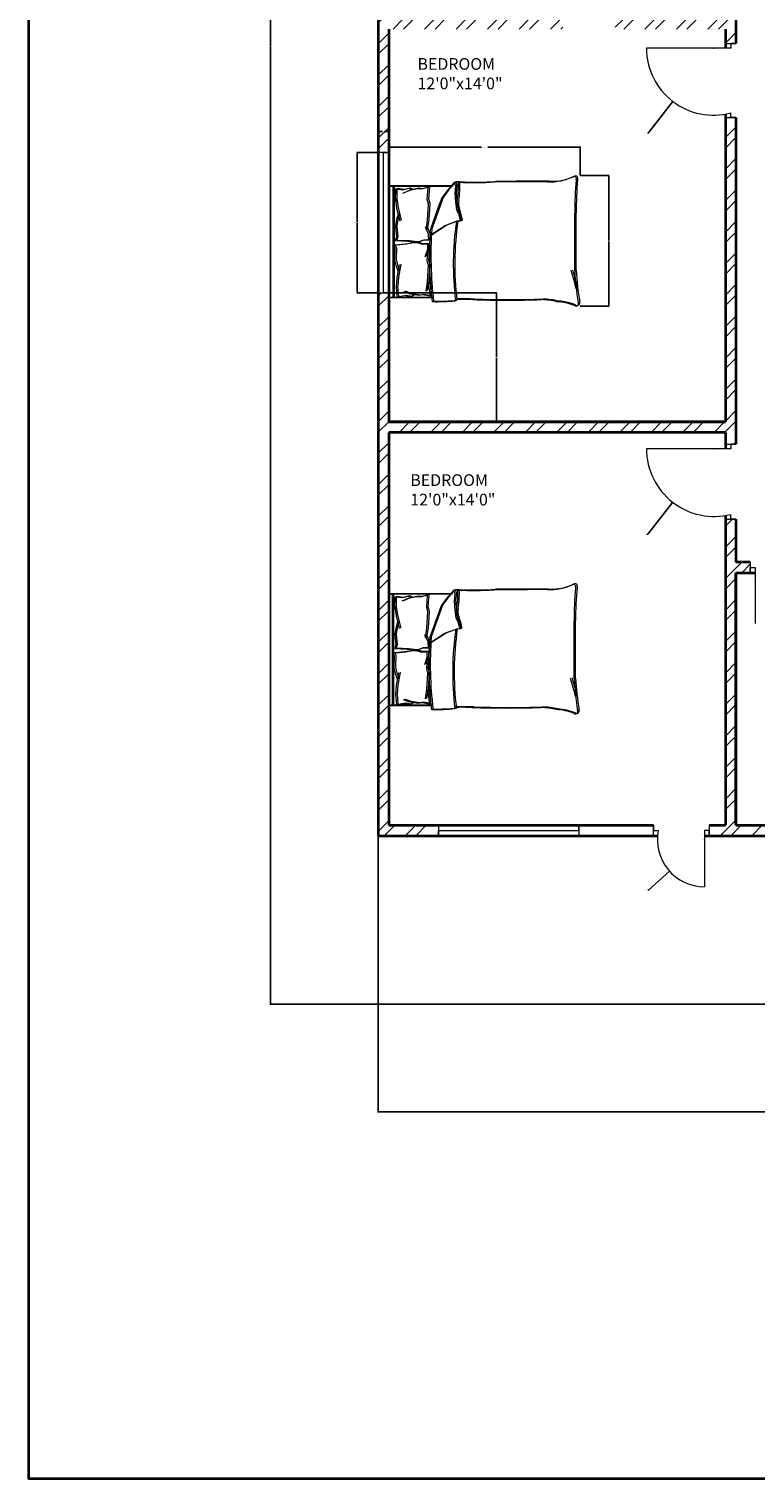
# Model space of a CAD drawing. Units: inches. Extents: x 392 to 1254, y 1207 to 2665.
# Tile 1 of 15: x 392 to 702, y 1207 to 1827. Entities that reach past the tile are written whole.
import ezdxf

# ---------------------------------------------------------------- set-up
doc = ezdxf.new("R2010")
doc.units = ezdxf.units.IN
for name, color, linetype, lineweight in [('A-ANNO-DIMS', 2, 'Continuous', 18), ('A-ANNO-TTLB', 7, 'Continuous', 35), ('A-AREA-IDEN', 7, 'Continuous', 18), ('A-DOOR', 3, 'Continuous', 18), ('A-FURN', 8, 'Continuous', 13), ('A-GLAZ', 4, 'Continuous', 18), ('A-WALL', 7, 'Continuous', 35), ('A-WALL-PATT', 252, 'Continuous', 13)]:
    doc.layers.add(name, color=color, linetype=linetype, lineweight=lineweight)
doc.styles.get("Standard").update_dxf_attribs({"font": 'arial.ttf'})
doc.dimstyles.get("Standard").update_dxf_attribs({"dimtxt": 0.18, "dimasz": 0.18, "dimexe": 0.18, "dimexo": 0.0625, "dimgap": 0.09, "dimtad": 0, "dimtih": 1, "dimtoh": 1, "dimdec": 4, "dimzin": 0, "dimdsep": 46, "dimtxsty": 'Standard', "dimcen": 0.09, "dimadec": 0, "dimazin": 0, "dimtfac": 1, "dimtdec": 4, "dimtofl": 0, "dimtmove": 0, "dimatfit": 3, "dimfxl": 1, "dimtolj": 1, "dimtzin": 0, "dimarcsym": 0})

# ---------------------------------------------------------------- blocks, each defined once
blk = doc.blocks.new('BED-DOUBLE')
for p, q in [((3.47, 63.33), (3.47, 81.44)), ((3.48, 63.33), (3.48, 81.44)), ((3.7, 62.69), (3.7, 80.8)), ((3.7, 62.69), (3.7, 80.8)), ((51.27, 81.44), (51.27, 54.83)), ((51.27, 81.44), (51.27, 54.83)), ((51.49, 81.44), (51.49, 80.8)), ((51.49, 80.8), (51.49, 54.19)), ((51.49, 80.8), (51.49, 54.19)), ((3.47, 79.91), (51.27, 79.91)), ((3.48, 79.91), (51.27, 79.91)), ((3.7, 79.27), (51.49, 79.27)), ((3.7, 79.27), (51.49, 79.27)), ((3.89, 78.13), (4.47, 74.95)), ((3.89, 78.13), (4.47, 74.95)), ((3.9, 78.1), (8.18, 78.43)), ((3.9, 78.1), (8.18, 78.43)), ((4.47, 74.95), (4.04, 72.34)), ((4.47, 74.95), (4.04, 72.34)), ((4.12, 77.49), (4.7, 74.31)), ((4.12, 77.49), (4.7, 74.31)), ((4.13, 77.47), (8.41, 77.79)), ((4.13, 77.47), (8.41, 77.79)), ((5.05, 72.49), (6.06, 75.23)), ((5.05, 72.49), (6.06, 75.23)), ((5.28, 71.85), (6.29, 74.6)), ((5.28, 71.85), (6.29, 74.6)), ((8.18, 78.43), (8.28, 78.42)), ((8.18, 78.43), (8.28, 78.42)), ((8.28, 78.42), (12.11, 78.13)), ((8.28, 78.42), (12.11, 78.13)), ((8.41, 77.79), (8.51, 77.78)), ((8.41, 77.79), (8.51, 77.78)), ((8.51, 77.78), (12.34, 77.49)), ((8.51, 77.78), (12.34, 77.49)), ((12.11, 78.13), (17.6, 77.11)), ((12.11, 78.13), (17.6, 77.11)), ((12.34, 77.49), (17.83, 76.48)), ((12.34, 77.49), (17.83, 76.48)), ((14.85, 77.69), (16.88, 78.42)), ((14.85, 77.69), (16.88, 78.42)), ((15.08, 77.05), (17.11, 77.78)), ((15.08, 77.05), (17.11, 77.78)), ((16.88, 78.42), (19.77, 79.14)), ((16.88, 78.42), (19.77, 79.14)), ((17.11, 77.78), (20, 78.5)), ((17.11, 77.78), (20, 78.5)), ((19.77, 79.14), (20.09, 79.14)), ((19.77, 79.14), (20.09, 79.14)), ((20, 78.5), (20.32, 78.5)), ((20, 78.5), (20.32, 78.5)), ((20.09, 79.14), (24.54, 78.99)), ((20.09, 79.14), (24.54, 78.99)), ((20.32, 78.5), (24.77, 78.35)), ((20.32, 78.5), (24.77, 78.35)), ((24.54, 78.99), (25.98, 79.57)), ((24.54, 78.99), (25.98, 79.57)), ((24.77, 78.35), (26.21, 78.93)), ((24.77, 78.35), (26.21, 78.93)), ((25.98, 79.57), (26.56, 74.22)), ((25.98, 79.57), (26.56, 74.22)), ((26.21, 78.93), (26.79, 73.58)), ((26.21, 78.93), (26.79, 73.58)), ((27.98, 78.95), (27.73, 73.58)), ((27.98, 78.95), (27.73, 73.58)), ((28.21, 78.31), (27.96, 72.94)), ((28.21, 78.31), (27.96, 72.94)), ((29.46, 78.46), (27.98, 78.95)), ((29.46, 78.46), (27.98, 78.95)), ((29.68, 77.82), (28.21, 78.31)), ((29.68, 77.82), (28.21, 78.31)), ((33.88, 78.89), (29.46, 78.46)), ((33.88, 78.89), (29.46, 78.46)), ((34.11, 78.25), (29.68, 77.82)), ((34.11, 78.25), (29.68, 77.82)), ((34.2, 78.91), (33.88, 78.89)), ((34.2, 78.91), (33.88, 78.89)), ((34.43, 78.27), (34.11, 78.25)), ((34.43, 78.27), (34.11, 78.25)), ((37.14, 78.36), (34.2, 78.91)), ((37.14, 78.36), (34.2, 78.91)), ((37.36, 77.73), (34.43, 78.27)), ((37.36, 77.73), (34.43, 78.27)), ((41.91, 78.37), (36.49, 77.02)), ((41.91, 78.37), (36.5, 77.02)), ((42.14, 77.73), (36.72, 76.38)), ((42.14, 77.73), (36.72, 76.38)), ((39.2, 77.77), (37.14, 78.36)), ((39.2, 77.77), (37.14, 78.36)), ((39.43, 77.13), (37.36, 77.73)), ((39.43, 77.13), (37.36, 77.73)), ((45.71, 78.9), (41.91, 78.37)), ((45.71, 78.9), (41.91, 78.37)), ((45.94, 78.26), (42.14, 77.73)), ((45.94, 78.26), (42.14, 77.73)), ((50.11, 78.89), (44.71, 78.98)), ((44.71, 78.98), (45.71, 78.9)), ((50.11, 78.89), (44.71, 78.98)), ((44.71, 78.98), (45.71, 78.9)), ((50.34, 78.25), (44.94, 78.34)), ((44.94, 78.34), (45.94, 78.26)), ((50.34, 78.25), (44.94, 78.34)), ((44.94, 78.34), (45.94, 78.26)), ((49.31, 73.19), (48.13, 75.86)), ((49.31, 73.19), (48.13, 75.86)), ((49.54, 72.55), (48.36, 75.22)), ((49.54, 72.55), (48.36, 75.22)), ((50.11, 78.89), (49.73, 75.67)), ((50.11, 78.89), (49.73, 75.67)), ((49.73, 75.67), (50.33, 73.1)), ((49.73, 75.67), (50.33, 73.1)), ((50.34, 78.25), (49.96, 75.04)), ((50.34, 78.25), (49.96, 75.04)), ((49.96, 75.04), (50.56, 72.47)), ((49.96, 75.04), (50.56, 72.47)), ((4.04, 72.34), (4.62, 71.33)), ((4.04, 72.34), (4.62, 71.33)), ((4.7, 74.31), (4.27, 71.7)), ((4.7, 74.31), (4.27, 71.7)), ((4.27, 71.7), (4.85, 70.69)), ((4.27, 71.7), (4.85, 70.69)), ((4.47, 68.87), (5.05, 72.49)), ((4.47, 68.87), (5.05, 72.49)), ((4.76, 67.28), (4.47, 68.87)), ((4.76, 67.28), (4.47, 68.87)), ((4.7, 68.23), (5.28, 71.85)), ((4.7, 68.23), (5.28, 71.85)), ((4.99, 66.64), (4.7, 68.23)), ((4.99, 66.64), (4.7, 68.23)), ((26.56, 74.22), (27.14, 71.04)), ((26.56, 74.22), (27.14, 71.04)), ((27.14, 69.74), (26.56, 67.86)), ((27.14, 69.74), (26.56, 67.86)), ((26.79, 73.58), (27.37, 70.4)), ((26.79, 73.58), (27.37, 70.4)), ((27.37, 69.1), (26.79, 67.22)), ((27.37, 69.1), (26.79, 67.22)), ((27.14, 71.04), (27.14, 69.74)), ((27.14, 71.04), (27.14, 69.74)), ((27.73, 73.58), (27.35, 70.36)), ((27.73, 73.58), (27.35, 70.36)), ((27.35, 70.36), (27.44, 69.07)), ((27.35, 70.36), (27.44, 69.07)), ((27.37, 70.4), (27.37, 69.1)), ((27.37, 70.4), (27.37, 69.1)), ((27.44, 69.07), (28.13, 67.23)), ((27.44, 69.07), (28.13, 67.23)), ((27.96, 72.94), (27.58, 69.73)), ((27.96, 72.94), (27.58, 69.73)), ((27.58, 69.73), (27.66, 68.43)), ((27.58, 69.73), (27.66, 68.43)), ((27.66, 68.43), (28.36, 66.59)), ((27.66, 68.43), (28.36, 66.59)), ((50.11, 69.61), (49.31, 73.19)), ((50.11, 69.61), (49.31, 73.19)), ((50.34, 68.97), (49.54, 72.55)), ((50.34, 68.97), (49.54, 72.55)), ((50.33, 73.1), (49.81, 72.06)), ((50.33, 73.1), (49.81, 72.06)), ((49.92, 68.01), (50.11, 69.61)), ((49.92, 68.01), (50.11, 69.61)), ((50.56, 72.47), (50.04, 71.42)), ((50.56, 72.47), (50.04, 71.42)), ((50.15, 67.37), (50.34, 68.97)), ((50.15, 67.37), (50.34, 68.97)), ((4.18, 64.1), (4.76, 67.28)), ((4.18, 64.1), (4.76, 67.28)), ((9.28, 64.82), (4.18, 64.1)), ((9.28, 64.82), (4.18, 64.1)), ((4.41, 63.46), (4.99, 66.64)), ((4.41, 63.46), (4.99, 66.64)), ((9.51, 64.19), (4.41, 63.46)), ((9.51, 64.19), (4.41, 63.46)), ((6.38, 65.81), (10.41, 65.15)), ((6.38, 65.81), (10.41, 65.15)), ((6.61, 65.17), (10.64, 64.51)), ((6.61, 65.17), (10.64, 64.51)), ((10.41, 65.15), (9.28, 64.82)), ((10.41, 65.15), (9.28, 64.82)), ((10.64, 64.51), (9.51, 64.19)), ((10.64, 64.51), (9.51, 64.19)), ((10.41, 65.15), (17.42, 64.72)), ((10.41, 65.15), (17.42, 64.72)), ((10.64, 64.51), (17.65, 64.08)), ((10.64, 64.51), (17.65, 64.08)), ((17.42, 64.72), (19.38, 65.27)), ((17.42, 64.72), (19.38, 65.27)), ((17.65, 64.08), (19.61, 64.63)), ((17.65, 64.08), (19.61, 64.63)), ((19.38, 65.27), (24.52, 64.87)), ((19.38, 65.27), (24.52, 64.87)), ((19.61, 64.63), (24.74, 64.23)), ((19.61, 64.63), (24.74, 64.23)), ((24.1, 65.18), (20.96, 66.27)), ((24.1, 65.18), (20.96, 66.27)), ((24.33, 64.54), (21.19, 65.63)), ((24.33, 64.54), (21.19, 65.63)), ((26.56, 65.18), (24.1, 65.18)), ((26.56, 65.18), (24.1, 65.18)), ((26.79, 64.54), (24.33, 64.54)), ((26.79, 64.54), (24.33, 64.54)), ((26.56, 67.86), (26.56, 65.18)), ((26.56, 67.86), (26.56, 65.18)), ((26.79, 67.22), (26.79, 64.54)), ((26.79, 67.22), (26.79, 64.54)), ((28.13, 67.23), (28.3, 64.55)), ((28.13, 67.23), (28.3, 64.55)), ((28.3, 64.55), (30.75, 64.7)), ((28.3, 64.55), (30.75, 64.7)), ((28.36, 66.59), (28.53, 63.91)), ((28.36, 66.59), (28.53, 63.91)), ((28.53, 63.91), (30.98, 64.06)), ((28.53, 63.91), (30.98, 64.06)), ((30.26, 64.06), (34.45, 57.57)), ((30.26, 64.06), (34.45, 57.57)), ((30.49, 63.42), (34.68, 56.93)), ((30.49, 63.42), (34.68, 56.93)), ((30.75, 64.7), (33.82, 65.99)), ((30.75, 64.7), (33.82, 65.99)), ((30.98, 64.06), (34.05, 65.35)), ((30.98, 64.06), (34.05, 65.35)), ((40.64, 61.13), (32.31, 64.06)), ((40.64, 61.13), (32.31, 64.06)), ((40.87, 60.49), (32.53, 63.42)), ((40.87, 60.49), (32.53, 63.42)), ((32.56, 65.81), (36.6, 65.15)), ((32.56, 65.81), (36.6, 65.15)), ((32.79, 65.17), (36.82, 64.51)), ((32.79, 65.17), (36.82, 64.51)), ((36.6, 65.15), (43.61, 64.72)), ((36.6, 65.15), (43.61, 64.72)), ((36.82, 64.51), (43.83, 64.08)), ((36.82, 64.51), (43.83, 64.08)), ((43.61, 64.72), (45.57, 65.27)), ((43.61, 64.72), (45.57, 65.27)), ((43.83, 64.08), (45.79, 64.63)), ((43.83, 64.08), (45.79, 64.63)), ((45.57, 65.27), (50.7, 64.87)), ((45.57, 65.27), (50.7, 64.87)), ((45.79, 64.63), (50.93, 64.23)), ((45.79, 64.63), (50.93, 64.23)), ((50.7, 64.87), (49.92, 68.01)), ((50.7, 64.87), (49.92, 68.01)), ((50.93, 64.23), (50.15, 67.37)), ((50.93, 64.23), (50.15, 67.37)), ((34.45, 57.57), (36.15, 53.08)), ((34.45, 57.57), (36.15, 53.08)), ((34.68, 56.93), (36.38, 52.44)), ((34.68, 56.93), (36.38, 52.44)), ((46.22, 59.11), (40.64, 61.13)), ((46.22, 59.11), (40.64, 61.13)), ((46.45, 58.47), (40.87, 60.49)), ((46.45, 58.47), (40.87, 60.49)), ((49.16, 56.95), (46.22, 59.11)), ((49.16, 56.95), (46.22, 59.11)), ((49.39, 56.31), (46.45, 58.47)), ((49.39, 56.31), (46.45, 58.47)), ((52.87, 53.7), (49.16, 56.95)), ((52.87, 53.7), (49.16, 56.95)), ((53.1, 53.06), (49.39, 56.31)), ((53.1, 53.06), (49.39, 56.31)), ((36.15, 53.08), (36.46, 51.07)), ((36.15, 53.08), (36.46, 51.07)), ((36.38, 52.44), (36.69, 50.43)), ((36.38, 52.44), (36.69, 50.43)), ((36.46, 51.07), (38.94, 51.68)), ((36.46, 51.07), (38.94, 51.68)), ((36.69, 50.43), (39.17, 51.05)), ((36.69, 50.43), (39.17, 51.05)), ((38.94, 51.68), (40.95, 52.61)), ((38.94, 51.68), (40.95, 52.61)), ((39.17, 51.05), (41.18, 51.97)), ((39.17, 51.05), (41.18, 51.97)), ((40.95, 52.61), (44.36, 53.08)), ((40.95, 52.61), (44.36, 53.08)), ((41.18, 51.97), (44.59, 52.44)), ((41.18, 51.97), (44.59, 52.44)), ((44.36, 53.08), (48.23, 53.39)), ((44.36, 53.08), (48.23, 53.39)), ((44.59, 52.44), (48.46, 52.75)), ((44.59, 52.44), (48.46, 52.75)), ((48.23, 53.39), (51.33, 53.08)), ((48.23, 53.39), (51.33, 53.08)), ((48.46, 52.75), (51.56, 52.44)), ((48.46, 52.75), (51.56, 52.44)), ((51.33, 53.08), (52.87, 53.7)), ((51.33, 53.08), (52.87, 53.7)), ((51.56, 52.44), (53.1, 53.06)), ((51.56, 52.44), (53.1, 53.06)), ((52.95, 51.95), (52.87, 53.7, 3.87)), ((52.95, 51.95), (52.87, 53.7, 3.87)), ((53.18, 51.31), (53.1, 53.06, 3.87)), ((53.18, 51.31), (53.1, 53.06, 3.87)), ((15.06, 2.2), (39.68, 2.2)), ((15.06, 2.2), (39.68, 2.2)), ((15.29, 1.56), (39.91, 1.56)), ((15.29, 1.56), (39.91, 1.56))]:
    blk.add_line(p, q)
for centre, radius, start, end in [((85.16, 61.35), 83.31, 178.72178, 185.60397), ((85.16, 61.35), 83.31, 178.72178, 185.60397), ((21.36, -100.61), 164.97, 86.08655, 96.78213), ((21.36, -100.61), 164.97, 86.08655, 96.78213), ((85.39, 60.71), 83.31, 178.72178, 185.60397), ((85.39, 60.71), 83.31, 178.72178, 185.60397), ((21.59, -101.25), 164.97, 86.08655, 96.78213), ((21.59, -101.25), 164.97, 86.08655, 96.78213), ((17.76, -74.87), 129.02, 81.78449, 96.90062), ((17.76, -74.87), 129.02, 81.78449, 96.90062), ((17.98, -75.51), 129.02, 81.78449, 96.90062), ((17.98, -75.51), 129.02, 81.78449, 96.90062), ((-167.31, 50.27), 170.11, 358.4762, 1.00819), ((-167.31, 50.27), 170.11, 358.4762, 1.00819), ((-167.08, 49.63), 170.11, 358.4762, 1.00819), ((-167.08, 49.63), 170.11, 358.4762, 1.00819), ((36.64, 51), 0.185, 160.24637, 271.13765), ((36.64, 51), 0.185, 160.24637, 271.13765), ((31.15, 79.96), 29.65, 280.66171, 289.88058), ((31.15, 79.96), 29.65, 280.66171, 289.88058), ((36.86, 50.36), 0.185, 160.24637, 271.13765), ((36.86, 50.36), 0.185, 160.24637, 271.13765), ((31.38, 79.32), 29.65, 280.66171, 289.88058), ((31.38, 79.32), 29.65, 280.66171, 289.88058), ((43.74, 46.38), 6.22, 78.6608, 113.73842), ((43.74, 46.38), 6.22, 78.6608, 113.73842), ((43.97, 45.74), 6.22, 78.6608, 113.73842), ((43.97, 45.74), 6.22, 78.6608, 113.73842), ((51.33, 88.1), 36.18, 259.87628, 272.56571), ((51.33, 88.1), 36.18, 259.87628, 272.56571), ((51.56, 87.46), 36.18, 259.87628, 272.56571), ((51.56, 87.46), 36.18, 259.87628, 272.56571), ((182.27, 45.13), 129.5, 176.97912, 183.83645), ((182.27, 45.13), 129.5, 176.97912, 183.83645), ((182.49, 44.49), 129.5, 176.97912, 183.83645), ((182.49, 44.49), 129.5, 176.97912, 183.83645), ((484.82, 30.83), 482.31, 178.22771, 181.71854), ((484.82, 30.83), 482.31, 178.22771, 181.71854), ((485.05, 30.19), 482.31, 178.22771, 181.71854), ((485.05, 30.19), 482.31, 178.22771, 181.71854), ((-4508.74, 13.62), 4561.86, 0.00217, 0.28689), ((-4508.74, 13.62), 4561.86, 0.00217, 0.28689), ((-4508.51, 12.98), 4561.86, 0.00217, 0.28689), ((-4508.52, 12.98), 4561.86, 0.00217, 0.28689), ((-26.9, 16.93), 29.63, 346.06484, 358.91125), ((-26.9, 16.93), 29.63, 346.06484, 358.91125), ((-26.67, 16.29), 29.63, 346.06484, 358.91125), ((-26.67, 16.29), 29.63, 346.06484, 358.91125), ((76.16, 12.78), 23.07, 177.47136, 206.46809), ((76.16, 12.78), 23.07, 177.47136, 206.46809), ((76.39, 12.14), 23.07, 177.47136, 206.46809), ((76.39, 12.14), 23.07, 177.47136, 206.46809), ((-21.66, 11.17), 23.56, 337.97508, 356.652), ((-21.66, 11.17), 23.56, 337.97508, 356.652), ((-21.43, 10.53), 23.56, 337.97508, 356.652), ((-21.43, 10.53), 23.56, 337.97508, 356.652), ((1.09, 1.72), 1.09, 146.17358, 293.47814), ((1.09, 1.72), 1.09, 146.17358, 293.47814), ((1.32, 1.09), 1.09, 146.17358, 293.47814), ((1.32, 1.09), 1.09, 146.17358, 293.47814), ((21.43, -119.39), 121.76, 92.99578, 99.40907), ((21.43, -119.39), 121.76, 92.99578, 99.40907), ((21.66, -120.03), 121.76, 92.99578, 99.40907), ((21.65, -120.03), 121.76, 92.99578, 99.40907), ((-17.22, 105.15), 106.46, 283.38322, 287.70533), ((-17.22, 105.15), 106.46, 283.38322, 287.70533), ((-16.99, 104.52), 106.46, 283.38322, 287.70533), ((-16.99, 104.52), 106.46, 283.38322, 287.70533), ((41.15, -130.83), 133.04, 84.4998, 90.63509), ((41.15, -130.83), 133.04, 84.4998, 90.63509), ((41.38, -131.47), 133.04, 84.4998, 90.63509), ((41.38, -131.47), 133.04, 84.4998, 90.63509), ((54.41, 2.57), 1.1, 242.65876, 356.02002), ((54.41, 2.57), 1.1, 242.65876, 356.02002), ((54.64, 1.93), 1.1, 242.65876, 356.02002), ((54.64, 1.93), 1.1, 242.65876, 356.02002)]:
    blk.add_arc(centre, radius, start, end)
blk = doc.blocks.new('WIN-60-A')
for p, q in [((0, 60), (4.5, 60)), ((4.5, 60), (2.25, 60)), ((2.25, 60), (2.25, 0)), ((2.25, 0), (0, 0)), ((0, 0), (4.5, 0))]:
    blk.add_line(p, q)
blk = doc.blocks.new('WIN-60-B')
for p, q in [((4.5, 60), (0, 60)), ((2.25, 0), (2.25, 60)), ((2.25, 60), (4.5, 60)), ((0, 0), (4.5, 0)), ((4.5, 0), (2.25, 0))]:
    blk.add_line(p, q)
blk = doc.blocks.new('*D9')
at = {"layer": 'A-ANNO-DIMS', "color": 0, "lineweight": -2, "transparency": 16777216}
for p, q in [((546.09, 1764.64), (546.09, 1776.99)), ((546.27, 1776.81), (585.49, 1776.81)), ((627.46, 1776.81), (588.23, 1776.81)), ((627.64, 1764.64), (627.64, 1776.99))]:
    blk.add_line(p, q, dxfattribs=at)
at = {"layer": 'A-ANNO-DIMS', "color": 0, "transparency": 16777216}
for points in [[(546.27, 1776.84), (546.27, 1776.78), (546.09, 1776.81)], [(627.46, 1776.84), (627.46, 1776.78), (627.64, 1776.81)]]:
    blk.add_solid(points, dxfattribs=at)
at = {"layer": 'Defpoints', "color": 0, "transparency": 16777216}
for p in [(546.09, 1776.81), (546.09, 1764.58), (627.64, 1764.58)]:
    blk.add_point(p, dxfattribs=at)
at = {"layer": 'A-ANNO-DIMS', "color": 0, "transparency": 16777216, "insert": (586.86, 1776.81), "char_height": 0.18, "attachment_point": 5}
blk.add_mtext('\\A1;DOUBLE BED 82 TYP.', dxfattribs=at)
blk = doc.blocks.new('*D10')
at = {"layer": 'A-ANNO-DIMS', "color": 0, "lineweight": -2, "transparency": 16777216}
for p, q in [((627.7, 1764.58), (640.05, 1764.58)), ((639.87, 1764.4), (639.87, 1736.85)), ((639.87, 1708.93), (639.87, 1736.48)), ((627.7, 1708.75), (640.05, 1708.75))]:
    blk.add_line(p, q, dxfattribs=at)
at = {"layer": 'A-ANNO-DIMS', "color": 0, "transparency": 16777216}
for points in [[(639.84, 1764.4), (639.9, 1764.4), (639.87, 1764.58)], [(639.84, 1708.93), (639.9, 1708.93), (639.87, 1708.75)]]:
    blk.add_solid(points, dxfattribs=at)
at = {"layer": 'Defpoints', "color": 0, "transparency": 16777216}
for p in [(627.64, 1764.58), (639.87, 1764.58), (627.64, 1708.75)]:
    blk.add_point(p, dxfattribs=at)
at = {"layer": 'A-ANNO-DIMS', "color": 0, "transparency": 16777216, "insert": (639.87, 1736.66), "char_height": 0.18, "attachment_point": 5}
blk.add_mtext('\\A1;56 TYP.', dxfattribs=at)
blk = doc.blocks.new('*D21')
at = {"layer": 'A-ANNO-DIMS', "color": 0, "lineweight": -2, "transparency": 16777216}
for p, q in [((541.22, 1774.47), (532.1, 1774.47)), ((532.28, 1774.29), (532.28, 1744.65)), ((532.28, 1714.65), (532.28, 1744.28)), ((541.22, 1714.47), (532.1, 1714.47))]:
    blk.add_line(p, q, dxfattribs=at)
at = {"layer": 'A-ANNO-DIMS', "color": 0, "transparency": 16777216}
for points in [[(532.25, 1774.29), (532.31, 1774.29), (532.28, 1774.47)], [(532.25, 1714.65), (532.31, 1714.65), (532.28, 1714.47)]]:
    blk.add_solid(points, dxfattribs=at)
at = {"layer": 'Defpoints', "color": 0, "transparency": 16777216}
for p in [(532.28, 1774.47), (541.28, 1774.47), (541.28, 1714.47)]:
    blk.add_point(p, dxfattribs=at)
at = {"layer": 'A-ANNO-DIMS', "color": 0, "transparency": 16777216, "insert": (532.28, 1744.47), "char_height": 0.18, "attachment_point": 5}
blk.add_mtext('\\A1;WINDOW B 60 TYP.', dxfattribs=at)
blk = doc.blocks.new('*D22')
at = {"layer": 'A-ANNO-DIMS', "color": 0, "lineweight": -2, "transparency": 16777216}
for p, q in [((541.28, 1774.53), (541.28, 1783.65)), ((541.46, 1783.47), (543.07, 1783.47)), ((545.6, 1783.47), (543.99, 1783.47)), ((545.78, 1774.53), (545.78, 1783.65))]:
    blk.add_line(p, q, dxfattribs=at)
at = {"layer": 'A-ANNO-DIMS', "color": 0, "transparency": 16777216}
for points in [[(541.46, 1783.5), (541.46, 1783.44), (541.28, 1783.47)], [(545.6, 1783.5), (545.6, 1783.44), (545.78, 1783.47)]]:
    blk.add_solid(points, dxfattribs=at)
at = {"layer": 'Defpoints', "color": 0, "transparency": 16777216}
for p in [(545.78, 1783.47), (541.28, 1774.47), (545.78, 1774.47)]:
    blk.add_point(p, dxfattribs=at)
at = {"layer": 'A-ANNO-DIMS', "color": 0, "transparency": 16777216, "insert": (543.53, 1783.47), "char_height": 0.18, "attachment_point": 5}
blk.add_mtext('\\A1;5 TYP.', dxfattribs=at)
blk = doc.blocks.new('*D25')
at = {"layer": 'A-ANNO-DIMS', "color": 0, "lineweight": -2, "transparency": 16777216}
for p, q in [((541.28, 1482.23), (541.28, 1364.02)), ((1124.78, 1482.23), (1124.78, 1364.02)), ((541.46, 1364.2), (832.64, 1364.2)), ((1124.6, 1364.2), (833.43, 1364.2))]:
    blk.add_line(p, q, dxfattribs=at)
at = {"layer": 'A-ANNO-DIMS', "color": 0, "transparency": 16777216}
for points in [[(541.46, 1364.23), (541.46, 1364.17), (541.28, 1364.2)], [(1124.6, 1364.23), (1124.6, 1364.17), (1124.78, 1364.2)]]:
    blk.add_solid(points, dxfattribs=at)
at = {"layer": 'Defpoints', "color": 0, "transparency": 16777216}
for p in [(541.28, 1482.3), (1124.78, 1482.3), (1124.78, 1364.2)]:
    blk.add_point(p, dxfattribs=at)
at = {"layer": 'A-ANNO-DIMS', "color": 0, "transparency": 16777216, "insert": (833.03, 1364.2), "char_height": 0.18, "attachment_point": 5}
blk.add_mtext('\\A1;583.5', dxfattribs=at)
blk = doc.blocks.new('*D26')
at = {"layer": 'A-ANNO-DIMS', "color": 0, "lineweight": -2, "transparency": 16777216}
for p, q in [((541.22, 2229.3), (495, 2229.3)), ((495.18, 2229.12), (495.18, 1819.98)), ((495.18, 1410.48), (495.18, 1819.61)), ((753.23, 1410.3), (495, 1410.3))]:
    blk.add_line(p, q, dxfattribs=at)
at = {"layer": 'A-ANNO-DIMS', "color": 0, "transparency": 16777216}
for points in [[(495.15, 2229.12), (495.21, 2229.12), (495.18, 2229.3)], [(495.15, 1410.48), (495.21, 1410.48), (495.18, 1410.3)]]:
    blk.add_solid(points, dxfattribs=at)
at = {"layer": 'Defpoints', "color": 0, "transparency": 16777216}
for p in [(495.18, 2229.3), (541.28, 2229.3), (753.29, 1410.3)]:
    blk.add_point(p, dxfattribs=at)
at = {"layer": 'A-ANNO-DIMS', "color": 0, "transparency": 16777216, "insert": (495.18, 1819.8), "char_height": 0.18, "attachment_point": 5}
blk.add_mtext('\\A1;819', dxfattribs=at)
blk = doc.blocks.new('*D29')
at = {"layer": 'A-ANNO-DIMS', "color": 0, "lineweight": -2, "transparency": 16777216}
for p, q in [((541.28, 1482.23), (541.28, 1364.02)), ((753.29, 1410.23), (753.29, 1364.02)), ((541.46, 1364.2), (647, 1364.2)), ((753.11, 1364.2), (647.57, 1364.2))]:
    blk.add_line(p, q, dxfattribs=at)
at = {"layer": 'A-ANNO-DIMS', "color": 0, "transparency": 16777216}
for points in [[(541.46, 1364.23), (541.46, 1364.17), (541.28, 1364.2)], [(753.11, 1364.23), (753.11, 1364.17), (753.29, 1364.2)]]:
    blk.add_solid(points, dxfattribs=at)
at = {"layer": 'Defpoints', "color": 0, "transparency": 16777216}
for p in [(541.28, 1482.3), (753.29, 1410.3), (753.29, 1364.2)]:
    blk.add_point(p, dxfattribs=at)
at = {"layer": 'A-ANNO-DIMS', "color": 0, "transparency": 16777216, "insert": (647.28, 1364.2), "char_height": 0.18, "attachment_point": 5}
blk.add_mtext('\\A1;212', dxfattribs=at)
blk = doc.blocks.new('*D38')
at = {"layer": 'A-ANNO-DIMS', "color": 0, "lineweight": -2, "transparency": 16777216}
for p, q in [((545.84, 1714.47), (592.06, 1714.47)), ((591.88, 1714.29), (591.88, 1687.06)), ((591.88, 1659.48), (591.88, 1686.7)), ((545.84, 1659.3), (592.06, 1659.3))]:
    blk.add_line(p, q, dxfattribs=at)
at = {"layer": 'A-ANNO-DIMS', "color": 0, "transparency": 16777216}
for points in [[(591.85, 1714.29), (591.91, 1714.29), (591.88, 1714.47)], [(591.85, 1659.48), (591.91, 1659.48), (591.88, 1659.3)]]:
    blk.add_solid(points, dxfattribs=at)
at = {"layer": 'Defpoints', "color": 0, "transparency": 16777216}
for p in [(545.78, 1714.47), (545.78, 1659.3), (591.88, 1659.3)]:
    blk.add_point(p, dxfattribs=at)
at = {"layer": 'A-ANNO-DIMS', "color": 0, "transparency": 16777216, "insert": (591.88, 1686.88), "char_height": 0.18, "attachment_point": 5}
blk.add_mtext('\\A1;55.17', dxfattribs=at)
blk = doc.blocks.new('*D87')
at = {"layer": 'A-ANNO-DIMS', "color": 0, "lineweight": -2, "transparency": 16777216}
for p, q in [((684.84, 1647.77), (685.02, 1647.77)), ((684.93, 1647.68), (684.93, 1647.86)), ((656.53, 1611.27), (667.07, 1624.82)), ((656.35, 1611.27), (656.53, 1611.27))]:
    blk.add_line(p, q, dxfattribs=at)
at = {"layer": 'A-ANNO-DIMS', "color": 0, "transparency": 16777216}
blk.add_solid([(667.05, 1624.84), (667.09, 1624.8), (667.18, 1624.96)], dxfattribs=at)
at = {"layer": 'Defpoints', "color": 0, "transparency": 16777216}
for p in [(684.93, 1647.77), (667.18, 1624.96)]:
    blk.add_point(p, dxfattribs=at)
at = {"layer": 'A-ANNO-DIMS', "color": 0, "transparency": 16777216, "insert": (655.8, 1611.27), "char_height": 0.18, "attachment_point": 5}
blk.add_mtext('\\A1;R28.904', dxfattribs=at)
blk = doc.blocks.new('*D89')
at = {"layer": 'A-ANNO-DIMS', "color": 0, "lineweight": -2, "transparency": 16777216}
for p, q in [((684.56, 1819.05), (684.74, 1819.05)), ((684.65, 1818.96), (684.65, 1819.14)), ((656.75, 1782.74), (667.11, 1796.21)), ((656.57, 1782.74), (656.75, 1782.74))]:
    blk.add_line(p, q, dxfattribs=at)
at = {"layer": 'A-ANNO-DIMS', "color": 0, "transparency": 16777216}
blk.add_solid([(667.08, 1796.23), (667.13, 1796.19), (667.22, 1796.36)], dxfattribs=at)
at = {"layer": 'Defpoints', "color": 0, "transparency": 16777216}
for p in [(684.65, 1819.05), (667.22, 1796.36)]:
    blk.add_point(p, dxfattribs=at)
at = {"layer": 'A-ANNO-DIMS', "color": 0, "transparency": 16777216, "insert": (656.1, 1782.74), "char_height": 0.18, "attachment_point": 5}
blk.add_mtext('\\A1;R28.62', dxfattribs=at)
blk = doc.blocks.new('*D103')
at = {"layer": 'A-ANNO-DIMS', "color": 0, "lineweight": -2, "transparency": 16777216}
for p, q in [((702.33, 1591.29), (702.51, 1591.29)), ((702.42, 1591.2), (702.42, 1591.38)), ((723.92, 1571.54), (715.99, 1578.83)), ((724.1, 1571.54), (723.92, 1571.54))]:
    blk.add_line(p, q, dxfattribs=at)
at = {"layer": 'A-ANNO-DIMS', "color": 0, "transparency": 16777216}
blk.add_solid([(716.01, 1578.85), (715.97, 1578.81), (715.86, 1578.95)], dxfattribs=at)
at = {"layer": 'Defpoints', "color": 0, "transparency": 16777216}
for p in [(702.42, 1591.29), (715.86, 1578.95)]:
    blk.add_point(p, dxfattribs=at)
at = {"layer": 'A-ANNO-DIMS', "color": 0, "transparency": 16777216, "insert": (724.65, 1571.54), "char_height": 0.18, "attachment_point": 5}
blk.add_mtext('\\A1;R18.247', dxfattribs=at)
blk = doc.blocks.new('*D105')
at = {"layer": 'A-ANNO-DIMS', "color": 0, "lineweight": -2, "transparency": 16777216}
for p, q in [((680.68, 1480.63), (680.86, 1480.63)), ((680.77, 1480.54), (680.77, 1480.72)), ((656.91, 1459.11), (665.72, 1467.06)), ((656.73, 1459.11), (656.91, 1459.11))]:
    blk.add_line(p, q, dxfattribs=at)
at = {"layer": 'A-ANNO-DIMS', "color": 0, "transparency": 16777216}
blk.add_solid([(665.7, 1467.08), (665.74, 1467.03), (665.85, 1467.18)], dxfattribs=at)
at = {"layer": 'Defpoints', "color": 0, "transparency": 16777216}
for p in [(680.77, 1480.63), (665.85, 1467.18)]:
    blk.add_point(p, dxfattribs=at)
at = {"layer": 'A-ANNO-DIMS', "color": 0, "transparency": 16777216, "insert": (656.18, 1459.11), "char_height": 0.18, "attachment_point": 5}
blk.add_mtext('\\A1;R20.084', dxfattribs=at)

msp = doc.modelspace()

# ---------------------------------------------------------------- hatches: boundary and pattern name
at = {"layer": 'A-WALL-PATT'}
h = msp.add_hatch(dxfattribs=at)
h.set_pattern_fill('ANSI32', color=256)
h.paths.add_polyline_path([(579.5309, 2227.0453), (579.5309, 2229.2953), (541.2807, 2229.2953), (541.2807, 2182.3091), (545.7807, 2182.3091), (545.7807, 2224.7953), (579.5309, 2224.7953)])
h.paths.add_polyline_path([(655.4442, 2229.2953), (627.5309, 2229.2953), (627.5309, 2224.7953), (655.4442, 2224.7953), (655.4442, 2227.0453)])
h.paths.add_polyline_path([(703.0758, 2229.2953), (678.5257, 2229.2953), (678.5257, 2227.0453), (678.5257, 2224.7953), (689.7807, 2224.7953), (689.7807, 2158.6973), (694.2807, 2158.6973), (694.2807, 2224.7953), (703.0758, 2224.7953)])
h.paths.add_polyline_path([(768.5767, 2229.2953), (727.0758, 2229.2953), (727.0758, 2224.7953), (742.2807, 2224.7953), (742.2807, 2128.7953), (694.2807, 2128.7953), (694.2807, 2134.0554), (689.7807, 2134.0554), (689.7807, 2090.2854), (694.2807, 2090.2854), (694.2807, 2124.2953), (742.2807, 2124.2953), (742.2807, 2052.2953), (795.2124, 2052.2953), (795.2124, 2054.5453), (795.2124, 2056.7953), (746.7807, 2056.7953), (746.7807, 2224.7953), (768.5767, 2224.7953)])
h.paths.add_polyline_path([(867.5089, 2229.2953), (804.5767, 2229.2953), (804.5767, 2224.7953), (830.7807, 2224.7953), (830.7807, 2056.7953), (826.9066, 2056.7953), (826.9066, 2052.2953), (830.7807, 2052.2953), (830.7807, 1886.6777, -0.01766664), (830.8602, 1884.2953), (835.0818, 1884.2953, -0.04411348), (835.2807, 1889.9369), (835.2807, 2052.2953), (839.418, 2052.2953), (839.418, 2056.7953), (835.2807, 2056.7953), (835.2807, 2224.7953), (867.5089, 2224.7953)])
h.paths.add_polyline_path([(939.8604, 2229.2953), (903.5089, 2229.2953), (903.5089, 2227.0453), (903.5089, 2224.7953), (919.2807, 2224.7953), (919.2807, 2056.7953), (870.6499, 2056.7953), (870.6499, 2052.2953), (923.7807, 2052.2953), (923.7807, 2124.2953), (971.7807, 2124.2953), (971.7807, 2089.7112), (974.0307, 2089.7112), (976.2807, 2089.7112), (976.2807, 2133.56), (974.0307, 2133.56), (971.7807, 2133.56), (971.7807, 2128.7953), (923.7807, 2128.7953), (923.7807, 2224.7953), (939.8604, 2224.7953)])
h.paths.add_polyline_path([(1124.7807, 2229.2953), (1009.403, 2229.2953), (1009.403, 2224.7953), (1120.2807, 2224.7953), (1120.2807, 2184.7605), (1124.7807, 2184.7605)])
h.paths.add_polyline_path([(1124.7807, 2124.7605), (1120.2807, 2124.7605), (1120.2807, 2056.7953), (976.2807, 2056.7953), (976.2807, 2061.471), (971.7807, 2061.471), (971.7807, 2047.7483), (974.0307, 2047.7483), (976.2807, 2047.7483), (976.2807, 2052.2953), (1120.2807, 2052.2953), (1120.2807, 1992.457), (1124.7807, 1992.457)])
h.paths.add_polyline_path([(1124.7807, 1932.457), (1122.5307, 1932.457), (1120.2807, 1932.457), (1120.2807, 1884.2953), (976.2807, 1884.2953), (976.2807, 2019.9536), (971.7807, 2019.9536), (971.7807, 1884.2953), (869.0911, 1884.2953), (869.0911, 1879.7953), (971.7807, 1879.7953), (1013.7807, 1879.7953), (1013.7807, 1831.7953), (971.7807, 1831.7953), (971.7807, 1822.3831), (974.0307, 1822.3831), (976.2807, 1822.3831), (976.2807, 1827.2953), (1013.7807, 1827.2953), (1025.6191, 1827.2953), (1025.6191, 1829.5453), (1025.6191, 1831.7953), (1018.2807, 1831.7953), (1018.2807, 1879.7953), (1120.2807, 1879.7953), (1120.2807, 1866.9192), (1124.7807, 1866.9192)])
h.paths.add_polyline_path([(1124.7807, 1842.9192), (1122.5307, 1842.9192), (1120.2807, 1842.9192), (1120.2807, 1831.7953), (1050.2021, 1831.7953), (1050.2021, 1827.2953), (1120.2807, 1827.2953), (1120.2807, 1781.4559), (1124.7807, 1781.4559)])
h.paths.add_polyline_path([(976.2807, 1790.8718), (971.7807, 1790.8718), (971.7807, 1648.3339), (976.2807, 1648.3339), (976.2807, 1654.7953), (1120.2807, 1654.7953), (1120.2807, 1626.3807), (1124.7807, 1626.3807), (1124.7807, 1721.4559), (1120.2807, 1721.4559), (1120.2807, 1659.2953), (976.2807, 1659.2953)])
h.paths.add_polyline_path([(1124.7807, 1566.3807), (1120.2807, 1566.3807), (1120.2807, 1486.7953), (1101.07, 1486.7953), (1101.07, 1482.2953), (1124.7807, 1482.2953)])
h.paths.add_polyline_path([(1041.07, 1484.5453), (1041.07, 1486.7953), (1006.2807, 1486.7953), (1006.2807, 1484.5453), (1006.2807, 1482.2953), (1041.07, 1482.2953)])
h.paths.add_polyline_path([(976.2807, 1617.5497), (974.0307, 1617.5497), (971.7807, 1617.5497), (971.7807, 1599.2953), (965.8041, 1599.2953), (965.8041, 1594.7953), (971.7807, 1594.7953), (971.7807, 1486.7953), (954.1249, 1486.7953), (954.1249, 1482.2953), (981.5717, 1482.2953), (981.5717, 1484.5453), (981.5717, 1486.7953), (976.2807, 1486.7953)])
h.paths.add_polyline_path([(930.1249, 1486.7953), (887.7807, 1486.7953), (887.7807, 1594.7953), (941.9141, 1594.7953), (941.9141, 1597.0453), (941.9141, 1599.2953), (887.7807, 1599.2953), (887.7807, 1659.2953), (863.5916, 1659.2953), (863.5916, 1654.7953), (883.2807, 1654.7953), (883.2807, 1438.7953), (782.7807, 1438.7953), (782.7807, 1486.7953), (782.7807, 1654.7953), (800.1309, 1654.7953), (800.1309, 1657.0453), (800.1309, 1659.2953), (778.2807, 1659.2953), (778.2807, 1599.2953), (721.7333, 1599.2953), (721.7333, 1597.0453), (721.7333, 1594.7953), (778.2807, 1594.7953), (778.2807, 1486.7953), (729.598, 1486.7953), (729.598, 1482.2953), (753.2885, 1482.2953), (753.2885, 1410.2953), (922.9852, 1410.2953), (922.9852, 1482.2953), (930.1249, 1482.2953)])
h.paths.add_polyline_path([(918.4852, 1482.2953), (918.4852, 1414.7953), (757.7885, 1414.7953), (757.7885, 1482.2953), (778.2807, 1482.2953), (778.2807, 1434.2953), (782.7807, 1434.2953), (887.7807, 1434.2953), (887.7807, 1438.7953), (887.7807, 1482.2953)], flags=16)
h.paths.add_polyline_path([(694.2807, 1594.7953), (700.4169, 1594.7953), (700.4169, 1597.0453), (700.4169, 1599.2953), (694.2807, 1599.2953), (694.2807, 1617.7503), (692.0307, 1617.7503), (689.7807, 1617.7503), (689.7807, 1486.7953), (682.7672, 1486.7953), (682.7672, 1482.2953), (705.598, 1482.2953), (705.598, 1484.5453), (705.598, 1486.7953), (694.2807, 1486.7953)])
h.paths.add_polyline_path([(545.7807, 1654.7953), (689.7807, 1654.7953), (689.7807, 1649.7691), (694.2807, 1649.7691), (694.2807, 1789.3981), (692.0307, 1789.3981), (689.7807, 1789.3981), (689.7807, 1659.2953), (545.7807, 1659.2953), (545.7807, 1714.4681), (543.5307, 1714.4681), (541.2807, 1714.4681), (541.2807, 1482.2953), (567.0628, 1482.2953), (567.0628, 1484.5453), (567.0628, 1486.7953), (545.7807, 1486.7953)])
h.paths.add_polyline_path([(545.7807, 1827.2953), (620.2247, 1827.2953), (620.2247, 1829.5453), (620.2247, 1831.7953), (545.7807, 1831.7953), (545.7807, 1846.8518), (541.2807, 1846.8518), (541.2807, 1774.4681), (545.7807, 1774.4681)])
h.paths.add_polyline_path([(797.0944, 1884.2953), (694.2807, 1884.2953), (694.2807, 2019.0288), (692.0307, 2019.0288), (689.7807, 2019.0288), (689.7807, 1884.2953), (545.7807, 1884.2953), (545.7807, 1951.8244), (541.2807, 1951.8244), (541.2807, 1870.8518), (543.5307, 1870.8518), (545.7807, 1870.8518), (545.7807, 1879.7953), (647.7807, 1879.7953), (647.7807, 1831.7953), (642.6413, 1831.7953), (642.6413, 1827.2953), (652.2807, 1827.2953), (689.7807, 1827.2953), (689.7807, 1821.0531), (694.2807, 1821.0531), (694.2807, 1831.7953), (652.2807, 1831.7953), (652.2807, 1879.7953), (797.0944, 1879.7953), (797.0944, 1882.0453)])
h.paths.add_polyline_path([(545.7807, 2122.3091), (541.2807, 2122.3091), (541.2807, 2011.8244), (543.5307, 2011.8244), (545.7807, 2011.8244), (545.7807, 2052.2953), (689.7807, 2052.2953), (689.7807, 2048.2048), (694.2807, 2048.2048), (694.2807, 2061.3129), (692.0307, 2061.3129), (689.7807, 2061.3129), (689.7807, 2056.7953), (545.7807, 2056.7953)])

# ---------------------------------------------------------------- linework, layer by layer
at = {"layer": 'A-ANNO-TTLB'}
msp.add_lwpolyline([(391.939, 2664.8979), (1253.97, 2664.8979), (1253.97, 1207.2611), (391.939, 1207.2611)], close=True, dxfattribs=at)
at = {"layer": 'A-DOOR'}
for p, q in [((692.0307, 1819.0531), (656.0307, 1819.0531)), ((689.7807, 1821.0531), (694.2807, 1821.0531)), ((694.2807, 1821.0531), (692.0307, 1821.0531)), ((692.0307, 1821.0531), (692.0307, 1819.0531)), ((689.7807, 1789.3981), (694.2807, 1789.3981)), ((692.0307, 1789.3981), (692.0307, 1791.3981)), ((694.2807, 1789.3981), (692.0307, 1789.3981)), ((689.7807, 1649.7691), (694.2807, 1649.7691)), ((694.2807, 1649.7691), (692.0307, 1649.7691)), ((692.0307, 1649.7691), (692.0307, 1647.7691)), ((692.0307, 1647.7691), (656.0307, 1647.7691)), ((692.0307, 1617.7503), (692.0307, 1619.7503)), ((689.7807, 1617.7503), (694.2807, 1617.7503)), ((694.2807, 1617.7503), (692.0307, 1617.7503)), ((700.4169, 1599.2953), (700.4169, 1594.7953)), ((700.4169, 1594.7953), (700.4169, 1597.0453)), ((700.4169, 1597.0453), (702.4169, 1597.0453)), ((702.4169, 1597.0453), (702.4169, 1573.0453)), ((659.068, 1482.2953), (659.068, 1486.7953)), ((659.068, 1486.7953), (659.068, 1484.5453)), ((659.068, 1484.5453), (661.068, 1484.5453)), ((682.7672, 1484.5453), (680.7672, 1484.5453)), ((680.7672, 1484.5453), (680.7672, 1460.5453)), ((682.7672, 1486.7953), (682.7672, 1482.2953)), ((682.7672, 1482.2953), (682.7672, 1484.5453))]:
    msp.add_line(p, q, dxfattribs=at)
for centre, radius, start, end in [((684.6529, 1819.0531), 28.6222, 180, 284.9374382), ((684.9342, 1647.7691), 28.9035, 180, 284.2127679), ((680.7672, 1480.6298), 20.0845, 168.7580654, 270)]:
    msp.add_arc(centre, radius, start, end, dxfattribs=at)
at = {"layer": 'A-WALL'}
for p, q in [((541.2807, 2229.2953), (541.2807, 1482.2953)), ((694.2807, 1831.7953), (694.2807, 1821.0531)), ((545.7807, 1827.2953), (545.7807, 1659.2953)), ((689.7807, 1827.2953), (689.7807, 1819.0531)), ((689.7807, 1790.894), (689.7807, 1659.2953)), ((694.2807, 1789.3981), (694.2807, 1649.7691)), ((545.7807, 1659.2953), (689.7807, 1659.2953)), ((689.7807, 1659.2953), (545.7807, 1659.2953)), ((689.7807, 1654.7953), (545.7807, 1654.7953)), ((545.7807, 1654.7953), (545.7807, 1486.7953)), ((689.7807, 1654.7953), (689.7807, 1647.7691)), ((689.7807, 1619.2748), (689.7807, 1486.7953)), ((694.2807, 1617.7503), (694.2807, 1599.2953)), ((700.4169, 1599.2953), (694.2807, 1599.2953)), ((694.2807, 1486.7953), (694.2807, 1594.7953)), ((694.2807, 1594.7953), (702.4169, 1594.7953)), ((694.2807, 1594.7953), (694.2807, 1486.7953)), ((541.2807, 1482.2953), (660.7518, 1482.2953)), ((545.7807, 1486.7953), (659.068, 1486.7953)), ((680.7672, 1482.2953), (753.2885, 1482.2953)), ((682.7672, 1486.7953), (689.7807, 1486.7953)), ((694.2807, 1486.7953), (778.2807, 1486.7953))]:
    msp.add_line(p, q, dxfattribs=at)

# ---------------------------------------------------------------- block references
at = {"layer": 'A-FURN', "rotation": 90}
for p in [(627.5316, 1708.8374), (627.2757, 1534.4364)]:
    msp.add_blockref('BED-DOUBLE', p, dxfattribs=at)
at = {"layer": 'A-GLAZ'}
msp.add_blockref('WIN-60-B', (541.281, 1714.468), dxfattribs=at)
at = {"layer": 'A-GLAZ', "extrusion": (0, 0, -1), "zscale": -1, "rotation": 270}
msp.add_blockref('WIN-60-A', (-627.0628, 1486.795), dxfattribs=at)

# ---------------------------------------------------------------- texts
at = {"layer": 'A-AREA-IDEN', "char_height": 5, "attachment_point": 1}
for width, insert in [(131.261292, (558.0854, 1814.8501)), (154.200271, (555.0207, 1636.8953))]:
    msp.add_mtext_dynamic_manual_height_columns('BEDROOM\\P12\'0"x14\'0"', width=width, gutter_width=12.5, heights=[0], dxfattribs=dict(at, insert=insert))

# ---------------------------------------------------------------- dimensions: what is measured, and where the dimension line sits
at = {"layer": 'A-ANNO-DIMS'}
for base, p1, p2, angle, override, picture, middle in [((495.1807, 2229.2953), (753.2885, 1410.2953), (541.2807, 2229.2953), 90, {"dimdec": 0, "dimlfac": 1, "dimrnd": 0, "dimzin": 0, "dimdsep": 46, "dimlunit": 2}, '*D26', (495.1807, 1819.7953)), ((591.8807, 1659.2953), (545.7807, 1714.4681), (545.7807, 1659.2953), 270, {"dimdec": 2, "dimlfac": 1, "dimrnd": 0, "dimzin": 0, "dimdsep": 46, "dimlunit": 2}, '*D38', (591.8807, 1686.8817))]:
    dim = msp.add_linear_dim(base=base, p1=p1, p2=p2, angle=angle, dimstyle='Standard', override=override, dxfattribs=at)
    dim.commit()
    dim.dimension.update_dxf_attribs({"geometry": picture, "text_midpoint": middle})
for center, mpoint, override, picture, middle in [((684.6529, 1819.0531), (667.2162, 1796.3553), {"dimdec": 2, "dimlfac": 1, "dimrnd": 0, "dimzin": 0, "dimdsep": 46, "dimlunit": 2}, '*D89', (656.0953, 1782.7366)), ((684.93422, 1647.76908), (667.18182, 1624.95976), {"dimdec": 3, "dimlfac": 1, "dimrnd": 0, "dimzin": 0, "dimdsep": 46, "dimlunit": 2}, '*D87', (655.80098, 1611.27417)), ((702.4169, 1591.2923), (715.8555, 1578.949), {"dimdec": 3, "dimlfac": 1, "dimrnd": 0, "dimzin": 0, "dimdsep": 46, "dimlunit": 2}, '*D103', (724.6484, 1571.543)), ((680.76716, 1480.6298), (665.85333, 1467.1775), {"dimdec": 3, "dimlfac": 1, "dimrnd": 0, "dimzin": 0, "dimdsep": 46, "dimlunit": 2}, '*D105', (656.17564, 1459.10613))]:
    dim = msp.add_radius_dim(center=center, mpoint=mpoint, dimstyle='Standard', override=override, dxfattribs=at)
    dim.commit()
    dim.dimension.update_dxf_attribs({"geometry": picture, "text_midpoint": middle, "dimtype": 164})
dim = msp.add_linear_dim(base=(545.7807091188, 1783.4681089676), p1=(541.2807091188, 1774.4681089676), p2=(545.7807091188, 1774.4681089676), text='<> TYP.', dimstyle='Standard', override={"dimdec": 0, "dimlfac": 1, "dimrnd": 0, "dimzin": 0, "dimdsep": 46, "dimlunit": 2}, dxfattribs=at)
dim.commit()
dim.dimension.update_dxf_attribs({"geometry": '*D22', "text_midpoint": (543.5307091188, 1783.4681089676)})
for base, p1, p2, angle, text, picture, middle in [((532.2807, 1774.4681), (541.2807, 1714.4681), (541.2807, 1774.4681), 90, 'WINDOW B <> TYP.', '*D21', (532.2807, 1744.4681)), ((546.0889, 1776.8079), (627.6375, 1764.5756), (546.0889, 1764.5756), 180, 'DOUBLE BED <> TYP.', '*D9', (586.8632, 1776.8079)), ((639.8698, 1764.5756), (627.6375, 1708.751), (627.6375, 1764.5756), 90, '<> TYP.', '*D10', (639.8698, 1736.6633))]:
    dim = msp.add_linear_dim(base=base, p1=p1, p2=p2, angle=angle, text=text, dimstyle='Standard', override={"dimdec": 0, "dimlfac": 1, "dimrnd": 0, "dimzin": 0, "dimdsep": 46, "dimlunit": 2}, dxfattribs=at)
    dim.commit()
    dim.dimension.update_dxf_attribs({"geometry": picture, "text_midpoint": middle})
for base, p2, override, picture, middle in [((1124.7807, 1364.1953), (1124.7807, 1482.2953), {"dimdec": 1, "dimlfac": 1, "dimrnd": 0, "dimzin": 0, "dimdsep": 46, "dimlunit": 2}, '*D25', (833.0307, 1364.1953)), ((753.2885, 1364.1953), (753.2885, 1410.2953), {"dimdec": 0, "dimlfac": 1, "dimrnd": 0, "dimzin": 0, "dimdsep": 46, "dimlunit": 2}, '*D29', (647.2846, 1364.1953))]:
    dim = msp.add_linear_dim(base=base, p1=(541.2807, 1482.2953), p2=p2, dimstyle='Standard', override=override, dxfattribs=at)
    dim.commit()
    dim.dimension.update_dxf_attribs({"geometry": picture, "text_midpoint": middle})

doc.saveas('drawing.dxf')
